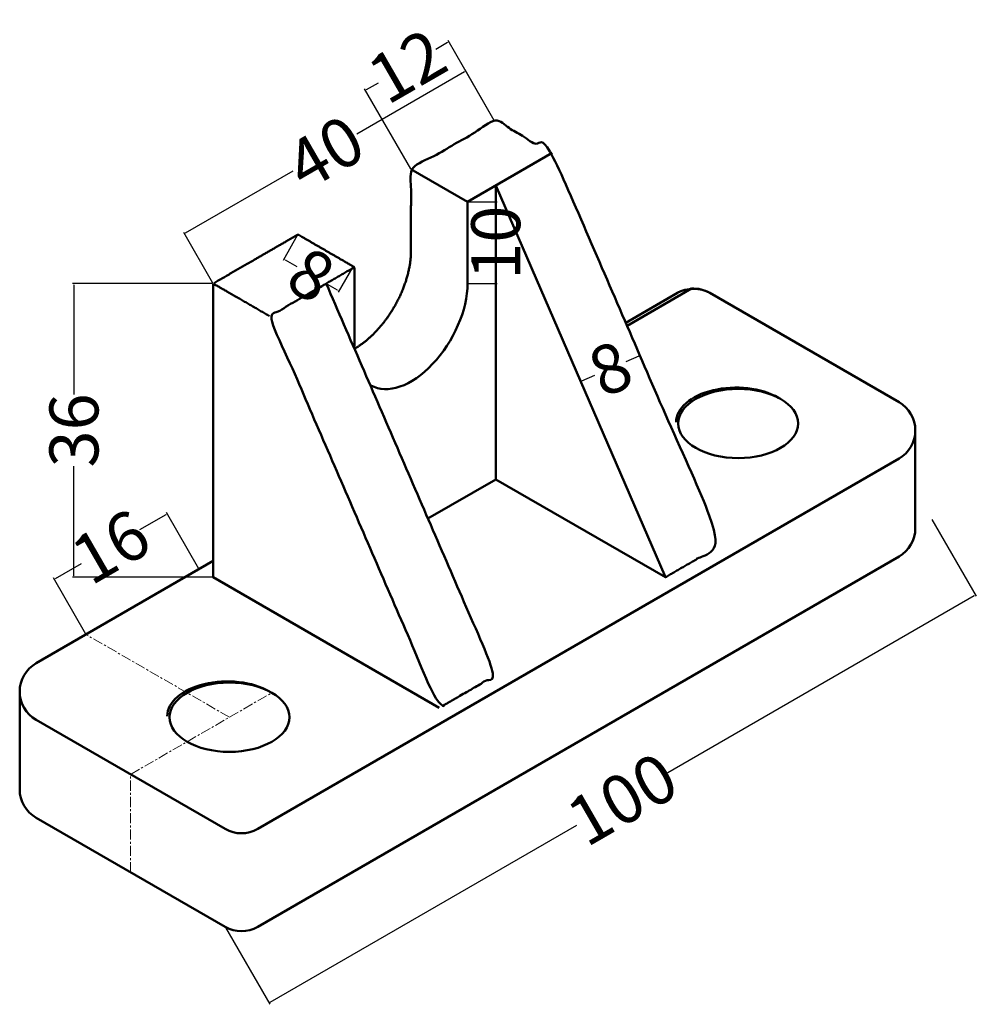
# Model space of a CAD drawing. Units: millimetres. Extents: x 5 to 123, y 36 to 156.
import ezdxf

# ---------------------------------------------------------------- set-up
doc = ezdxf.new("R2010")
doc.units = ezdxf.units.MM
doc.header["$MEASUREMENT"] = 0
doc.linetypes.add('CENTER', pattern=[2, 1.25, -0.25, 0.25, -0.25])
for name, color, linetype, lineweight in [('M-CNTR', 1, 'CENTER', 18), ('M-DIMS', 2, 'Continuous', 25), ('M-OUTL', 7, 'Continuous', 50)]:
    doc.layers.add(name, color=color, linetype=linetype, lineweight=lineweight)
doc.styles.get("Standard").update_dxf_attribs({"font": 'arial.ttf'})
doc.dimstyles.get("Standard").update_dxf_attribs({"dimtxt": 6, "dimasz": 0.18, "dimexe": 0.18, "dimexo": 0.0625, "dimgap": 0.09, "dimtad": 0, "dimtoh": 1, "dimdec": 0, "dimzin": 0, "dimdsep": 46, "dimtxsty": 'Standard', "dimcen": 0.09, "dimadec": 0, "dimazin": 0, "dimtfac": 1, "dimtdec": 0, "dimtofl": 0, "dimtmove": 0, "dimatfit": 3, "dimfxl": 1, "dimtolj": 1, "dimtzin": 0, "dimarcsym": 0})

# ---------------------------------------------------------------- blocks, each defined once
blk = doc.blocks.new('*D1')
at = {"layer": 'Defpoints', "color": 0, "transparency": 16777216}
for p in [(60.01, 150.09), (63.53, 143.98), (29.04, 124.07)]:
    blk.add_point(p, dxfattribs=at)
at = {"layer": 'M-DIMS', "color": 0, "lineweight": -2, "transparency": 16777216}
for p, q in [((59.85, 150), (46.66, 142.38)), ((63.5, 144.04), (59.92, 150.25)), ((25.67, 130.27), (38.87, 137.88)), ((29.01, 124.12), (25.43, 130.33))]:
    blk.add_line(p, q, dxfattribs=at)
at = {"layer": 'M-DIMS', "color": 0, "transparency": 16777216}
for points in [[(59.84, 150.03), (59.87, 149.97), (60.01, 150.09)], [(25.66, 130.29), (25.69, 130.24), (25.52, 130.18)]]:
    blk.add_solid(points, dxfattribs=at)
at = {"layer": 'M-DIMS', "color": 0, "transparency": 16777216, "insert": (42.76, 140.13), "char_height": 6, "attachment_point": 5, "rotation": 30}
blk.add_mtext('\\A1;40', dxfattribs=at)
blk = doc.blocks.new('*D2')
at = {"layer": 'Defpoints', "color": 0, "transparency": 16777216}
for p in [(60.22, 134.07), (60.22, 124.07), (63.68, 124.07)]:
    blk.add_point(p, dxfattribs=at)
at = {"layer": 'M-DIMS', "color": 0, "lineweight": -2, "transparency": 16777216}
for p, q in [((60.28, 134.07), (63.86, 134.07)), ((63.68, 133.89), (63.68, 133.17)), ((63.68, 124.25), (63.68, 124.98)), ((60.28, 124.07), (63.86, 124.07))]:
    blk.add_line(p, q, dxfattribs=at)
at = {"layer": 'M-DIMS', "color": 0, "transparency": 16777216}
for points in [[(63.65, 133.89), (63.71, 133.89), (63.68, 134.07)], [(63.65, 124.25), (63.71, 124.25), (63.68, 124.07)]]:
    blk.add_solid(points, dxfattribs=at)
at = {"layer": 'M-DIMS', "color": 0, "transparency": 16777216, "insert": (63.68, 129.07), "char_height": 6, "attachment_point": 5, "rotation": 90}
blk.add_mtext('\\A1;10', dxfattribs=at)
blk = doc.blocks.new('*D3')
at = {"layer": 'Defpoints', "color": 0, "transparency": 16777216}
for p in [(39.44, 130.07), (46.18, 126.18), (44.44, 123.18)]:
    blk.add_point(p, dxfattribs=at)
at = {"layer": 'M-DIMS', "color": 0, "lineweight": -2, "transparency": 16777216}
for p, q in [((39.4, 130.02), (37.61, 126.91)), ((37.86, 126.98), (39.28, 126.16)), ((46.15, 126.12), (44.35, 123.02)), ((44.29, 123.27), (42.86, 124.09))]:
    blk.add_line(p, q, dxfattribs=at)
at = {"layer": 'M-DIMS', "color": 0, "transparency": 16777216}
for points in [[(37.87, 127.01), (37.84, 126.95), (37.7, 127.07)], [(44.3, 123.29), (44.27, 123.24), (44.44, 123.18)]]:
    blk.add_solid(points, dxfattribs=at)
at = {"layer": 'M-DIMS', "color": 0, "transparency": 16777216, "insert": (41.07, 125.12), "char_height": 6, "attachment_point": 5, "rotation": 330}
blk.add_mtext('\\A1;8', dxfattribs=at)
blk = doc.blocks.new('*D4')
at = {"layer": 'Defpoints', "color": 0, "transparency": 16777216}
for p in [(81.37, 115.23), (81.37, 115.23), (74.08, 112.07)]:
    blk.add_point(p, dxfattribs=at)
at = {"layer": 'M-DIMS', "color": 0, "lineweight": -2, "transparency": 16777216}
for p, q in [((81.2, 115.16), (79.62, 114.47)), ((81.34, 115.29), (81.3, 115.39)), ((74.05, 112.13), (74, 112.24)), ((74.24, 112.14), (75.83, 112.83))]:
    blk.add_line(p, q, dxfattribs=at)
at = {"layer": 'M-DIMS', "color": 0, "transparency": 16777216}
for points in [[(81.19, 115.18), (81.22, 115.13), (81.37, 115.23)], [(74.23, 112.17), (74.25, 112.11), (74.08, 112.07)]]:
    blk.add_solid(points, dxfattribs=at)
at = {"layer": 'M-DIMS', "color": 0, "transparency": 16777216, "insert": (77.72, 113.65), "char_height": 6, "attachment_point": 5, "rotation": 23.4132}
blk.add_mtext('\\A1;8', dxfattribs=at)
blk = doc.blocks.new('*D5')
at = {"layer": 'Defpoints', "color": 0, "transparency": 16777216}
for p in [(117.11, 95.23), (122.49, 85.9), (30.51, 45.23)]:
    blk.add_point(p, dxfattribs=at)
at = {"layer": 'M-DIMS', "color": 0, "lineweight": -2, "transparency": 16777216}
for p, q in [((117.14, 95.17), (122.58, 85.74)), ((122.34, 85.81), (84.76, 64.11)), ((36.05, 35.99), (73.63, 57.68)), ((30.54, 45.17), (35.98, 35.74))]:
    blk.add_line(p, q, dxfattribs=at)
at = {"layer": 'M-DIMS', "color": 0, "transparency": 16777216}
for points in [[(122.32, 85.83), (122.35, 85.78), (122.49, 85.9)], [(36.03, 36.01), (36.06, 35.96), (35.89, 35.9)]]:
    blk.add_solid(points, dxfattribs=at)
at = {"layer": 'M-DIMS', "color": 0, "transparency": 16777216, "insert": (79.19, 60.9), "char_height": 6, "attachment_point": 5, "rotation": 30}
blk.add_mtext('\\A1;100', dxfattribs=at)
blk = doc.blocks.new('*D6')
at = {"layer": 'Defpoints', "color": 0, "transparency": 16777216}
for p in [(57.94, 153.68), (63.53, 143.98), (53.29, 138.07)]:
    blk.add_point(p, dxfattribs=at)
at = {"layer": 'M-DIMS', "color": 0, "lineweight": -2, "transparency": 16777216}
for p, q in [((57.78, 153.59), (56.35, 152.76)), ((63.5, 144.04), (57.85, 153.83)), ((47.85, 147.85), (49.29, 148.68)), ((53.26, 138.12), (47.61, 147.92))]:
    blk.add_line(p, q, dxfattribs=at)
at = {"layer": 'M-DIMS', "color": 0, "transparency": 16777216}
for points in [[(57.77, 153.61), (57.8, 153.56), (57.94, 153.68)], [(47.84, 147.88), (47.87, 147.83), (47.7, 147.76)]]:
    blk.add_solid(points, dxfattribs=at)
at = {"layer": 'M-DIMS', "color": 0, "transparency": 16777216, "insert": (52.82, 150.72), "char_height": 6, "attachment_point": 5, "rotation": 30}
blk.add_mtext('\\A1;12', dxfattribs=at)
blk = doc.blocks.new('*D7')
at = {"layer": 'Defpoints', "color": 0, "transparency": 16777216}
for p in [(29.04, 124.07), (11.98, 88.07), (29.04, 88.07)]:
    blk.add_point(p, dxfattribs=at)
at = {"layer": 'M-DIMS', "color": 0, "lineweight": -2, "transparency": 16777216}
for p, q in [((28.98, 124.07), (11.8, 124.07)), ((11.98, 123.89), (11.98, 110.45)), ((11.98, 88.25), (11.98, 101.69)), ((28.98, 88.07), (11.8, 88.07))]:
    blk.add_line(p, q, dxfattribs=at)
at = {"layer": 'M-DIMS', "color": 0, "transparency": 16777216}
for points in [[(11.95, 123.89), (12.01, 123.89), (11.98, 124.07)], [(11.95, 88.25), (12.01, 88.25), (11.98, 88.07)]]:
    blk.add_solid(points, dxfattribs=at)
at = {"layer": 'M-DIMS', "color": 0, "transparency": 16777216, "insert": (11.98, 106.07), "char_height": 6, "attachment_point": 5, "rotation": 90}
blk.add_mtext('\\A1;36', dxfattribs=at)
blk = doc.blocks.new('*D8')
at = {"layer": 'Defpoints', "color": 0, "transparency": 16777216}
for p in [(23.41, 95.83), (27.31, 89.07), (13.45, 81.07)]:
    blk.add_point(p, dxfattribs=at)
at = {"layer": 'M-DIMS', "color": 0, "lineweight": -2, "transparency": 16777216}
for p, q in [((23.25, 95.74), (20.03, 93.88)), ((27.28, 89.12), (23.32, 95.99)), ((9.71, 87.92), (12.92, 89.78)), ((13.42, 81.12), (9.46, 87.99))]:
    blk.add_line(p, q, dxfattribs=at)
at = {"layer": 'M-DIMS', "color": 0, "transparency": 16777216}
for points in [[(23.24, 95.77), (23.27, 95.72), (23.41, 95.83)], [(9.69, 87.95), (9.72, 87.9), (9.55, 87.83)]]:
    blk.add_solid(points, dxfattribs=at)
at = {"layer": 'M-DIMS', "color": 0, "transparency": 16777216, "insert": (16.48, 91.83), "char_height": 6, "attachment_point": 5, "rotation": 30}
blk.add_mtext('\\A1;16', dxfattribs=at)

msp = doc.modelspace()

# ---------------------------------------------------------------- linework, layer by layer
at = {"layer": 'M-CNTR'}
msp.add_line((31.04, 70.92), (13.45, 81.07), dxfattribs=at)
msp.add_lwpolyline([(18.92, 51.92), (18.92, 63.92), (36.24, 73.92)], dxfattribs=at)
at = {"layer": 'M-OUTL'}
for p, q in [((60.22, 134.07), (53.29, 138.07)), ((79.62, 119.27), (85.94, 122.92))]:
    msp.add_line(p, q, dxfattribs=at)
for points in [[(70.61, 140.07), (60.22, 134.07), (60.22, 124.07)], [(63.68, 100.07), (84.47, 88.07), (63.68, 136.07), (63.68, 100.07), (55.37, 95.27)], [(29.04, 124.07), (29.04, 88.07), (56.76, 72.07)]]:
    msp.add_lwpolyline(points, dxfattribs=at)
for points in [[(79.79, 118.89), (87.68, 123.44, -0.147669), (89.93, 122.92), (113.11, 109.53, -0.57735), (113.11, 102.61), (34.51, 57.23, -0.267949), (30.51, 57.23), (7.33, 70.61, -0.57735), (7.33, 77.53), (29.04, 90.07)], [(5.33, 74.07), (5.33, 62.07, 0.267949), (7.33, 58.61), (30.51, 45.23, 0.267949), (34.51, 45.23), (113.11, 90.61, 0.267949), (115.11, 94.07), (115.11, 106.07)]]:
    msp.add_lwpolyline(points, format="xyb", dxfattribs=at)
for centre, major_axis, start_param, end_param in [((53.29, 120.07), (-4.9, -8.49), 0, 2.356194), ((87.93, 121.77), (2.82, 0), 0.785398, 2.356194), ((93.13, 107.07), (7.35, 0), 0.785398, 3.141593), ((30.77, 71.07), (7.35, 0), 0.785398, 3.141593)]:
    msp.add_ellipse(centre, major_axis=major_axis, ratio=0.57735, start_param=start_param, end_param=end_param, dxfattribs=at)
for centre in [(93.4, 106.92), (31.04, 70.92)]:
    msp.add_ellipse(centre, major_axis=(-7.35, 0), ratio=0.57735, dxfattribs=at)
msp.add_rational_spline([(35.97, 120.07), (32.51, 122.07), (29.04, 124.07), (34.24, 127.07), (39.44, 130.07), (42.9, 128.07), (46.36, 126.07), (46.36, 121.07), (46.36, 116.07), (49.23, 117.73), (51.26, 121.24), (53.29, 124.76), (53.29, 128.07), (53.29, 133.07), (53.29, 138.07), (58.49, 141.07), (63.68, 144.07), (67.15, 142.07), (70.61, 140.07), (81, 116.07), (91.4, 92.07), (87.93, 90.07), (84.47, 88.07)], [1, 1, 1, 1, 1, 1, 1, 1, 1, 0.923879532511, 1, 0.923879532511, 1, 1, 1, 1, 1, 1, 1, 1, 1, 1, 1], degree=2, knots=[0, 0, 0, 1, 1, 2, 2, 3, 3, 4, 4, 4.785398, 4.785398, 5.570796, 5.570796, 6.570796, 6.570796, 7.570796, 7.570796, 8.570796, 8.570796, 9.570796, 9.570796, 10.570796, 10.570796, 10.570796], dxfattribs=at)
msp.add_open_spline([(46.36, 126.07), (41.17, 123.07), (35.97, 120.07), (46.36, 96.07), (56.76, 72.07), (60.22, 74.07), (63.68, 76.07), (53.29, 100.07), (42.9, 124.07)], degree=2, knots=[0, 0, 0, 1, 1, 2, 2, 3, 3, 4, 4, 4], dxfattribs=at)

# ---------------------------------------------------------------- dimensions: what is measured, and where the dimension line sits
at = {"layer": 'M-DIMS'}
for p1, p2, distance, picture, middle in [((53.29, 138.07), (63.53, 143.98), 11.19, '*D6', (52.82, 150.72)), ((29.04, 124.07), (63.53, 143.98), 7.05, '*D1', (42.76, 140.13)), ((60.22, 134.07), (60.22, 124.07), 3.46, '*D2', (63.68, 129.07)), ((39.44, 130.07), (46.18, 126.18), -3.46, '*D3', (41.07, 125.12)), ((29.04, 124.07), (29.04, 88.07), -17.06, '*D7', (11.98, 106.07)), ((74.08, 112.07), (81.37, 115.23), 0, '*D4', (77.72, 113.65)), ((13.45, 81.07), (27.31, 89.07), 7.81, '*D8', (16.48, 91.83)), ((30.51, 45.23), (117.11, 95.23), -10.77, '*D5', (79.19, 60.9))]:
    dim = msp.add_aligned_dim(p1=p1, p2=p2, distance=distance, dimstyle='Standard', override={"dimclrd": 0, "dimclre": 0, "dimclrt": 0}, dxfattribs=at)
    dim.commit()
    dim.dimension.update_dxf_attribs({"geometry": picture, "text_midpoint": middle})

doc.saveas('drawing.dxf')
